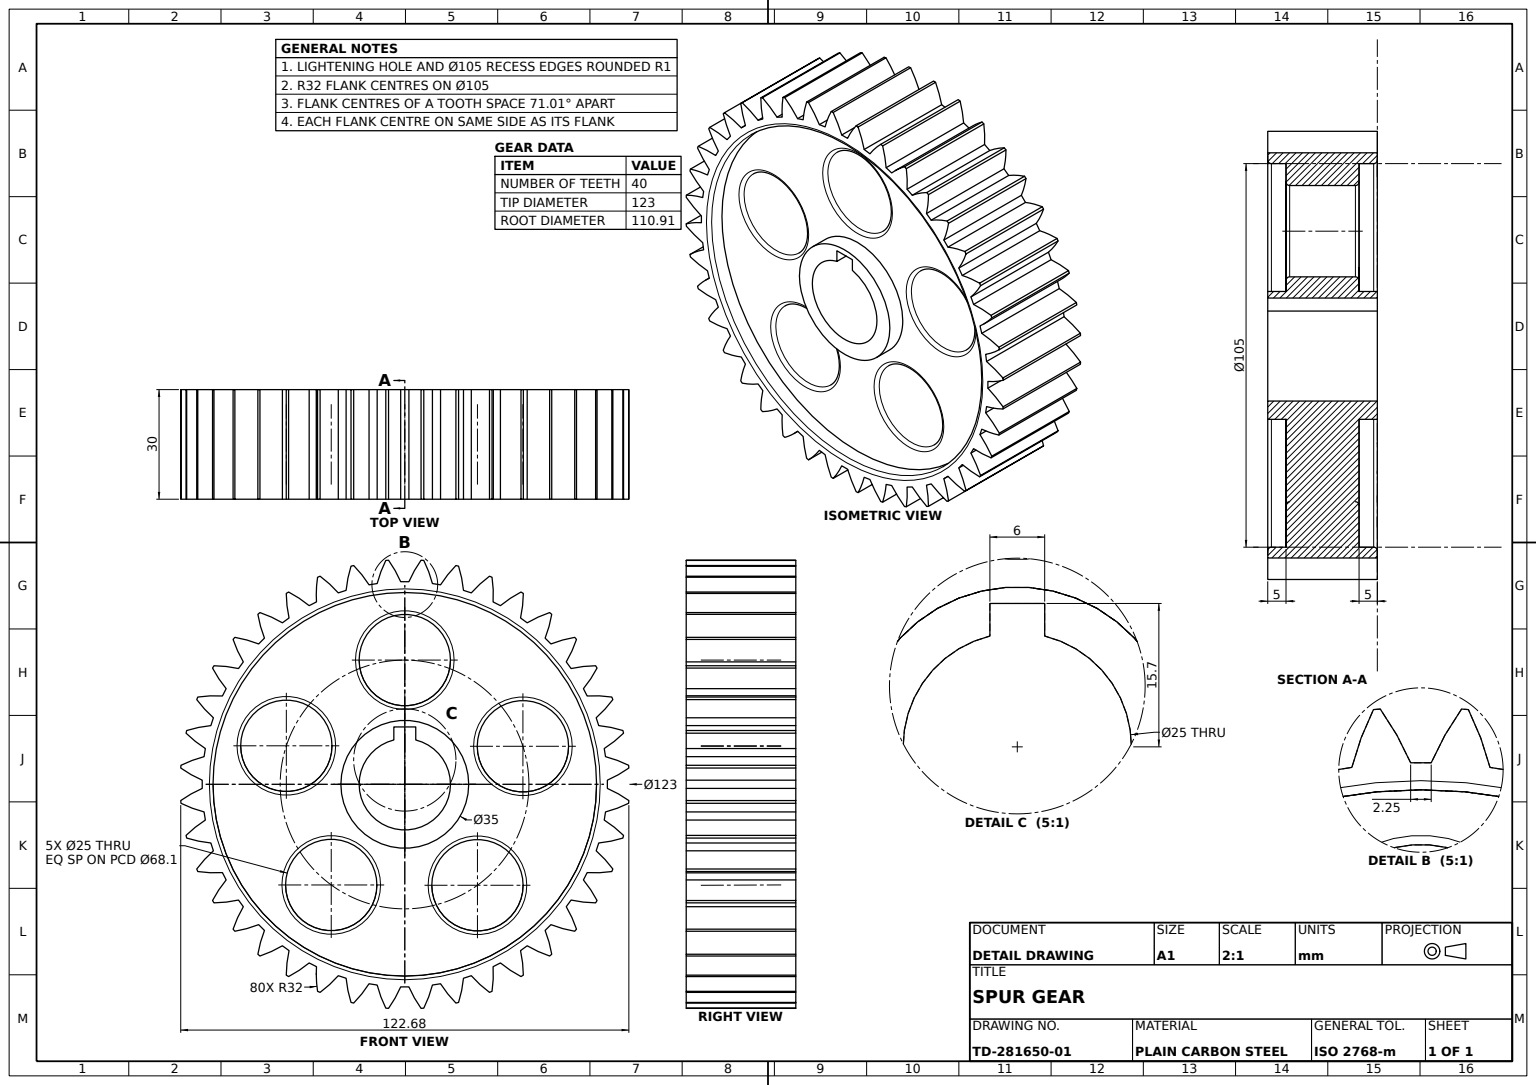
from build123d import *

# Parameters (mm, degrees)
GEAR_BLANK_SKETCH_R           = 61.5
GEAR_BLANK_DEPTH              = 30
FACE_RECESS_SKETCH_R          = 52.5
FACE_RECESS_105_DEPTH         = 5
TOOTH_SPACE_CUT_DEPTH         = 91.495856259
TOOTH_SPACE_PATTERN_40X_COUNT = 40
HUB_BOSS_SKETCH_R             = 17.5
HUB_BOSS_35_DEPTH             = 5
LIGHTENING_HOLES_DEPTH        = 91.276768883
LIGHTENING_HOLES_DEPTH_BACK   = 91.276768883
LIGHTENING_HOLES_SKETCH_R     = 12.5
EDGE_FILLETS_R1_R             = 1


with BuildPart() as part:
    # Gear Blank Sketch → Gear Blank (new body)
    with BuildSketch(Plane.XY):
        Circle(GEAR_BLANK_SKETCH_R)
        with BuildLine():
            Line((-3, 12.1346611), (-3, 15.7))
            Line((-3, 15.7), (3, 15.7))
            Line((3, 15.7), (3, 12.1346611))
            ThreePointArc((3, 12.1346611), (0, -12.5), (-3, 12.1346611))
        make_face(mode=Mode.SUBTRACT)
    extrude(amount=GEAR_BLANK_DEPTH)

    # Face Recess Sketch → Face Recess Ø105 (cut)
    with BuildSketch(Plane.XY.offset(30)):
        Circle(FACE_RECESS_SKETCH_R)
    face_recess_105 = extrude(amount=-FACE_RECESS_105_DEPTH, mode=Mode.SUBTRACT)

    # Face Recess Mirror: Face Recess Ø105 across plane
    add(face_recess_105.mirror(Plane.XY.offset(15)), mode=Mode.SUBTRACT)

    # Tooth Space Sketch → Tooth Space Cut (cut, symmetric)
    with BuildSketch(Plane.XY.offset(25)):
        with BuildLine():
            Line((-1.125, 55.456369197), (1.125, 55.456369197))
            ThreePointArc((1.125, 55.456369197), (2.631798544, 58.485590181), (4.45, 61.338792782))
            ThreePointArc((4.45, 61.338792782), (0, 61.5), (-4.45, 61.338792782))
            ThreePointArc((-4.45, 61.338792782), (-2.631798544, 58.485590181), (-1.125, 55.456369197))
        make_face()
    tooth_space_cut = extrude(amount=TOOTH_SPACE_CUT_DEPTH, both=True, mode=Mode.SUBTRACT)

    # Tooth Space Pattern 40x: Tooth Space Cut ×40 about axis
    tooth_space_pattern_40x_axis = Axis((0, 0, 0), (0, 0, 1))
    for i in range(1, TOOTH_SPACE_PATTERN_40X_COUNT):
        add(tooth_space_cut.rotate(tooth_space_pattern_40x_axis, i * 360 / TOOTH_SPACE_PATTERN_40X_COUNT), mode=Mode.SUBTRACT)

    # Hub Boss Sketch → Hub Boss Ø35 (add)
    with BuildSketch(Plane.XY.offset(25)):
        Circle(HUB_BOSS_SKETCH_R)
        with BuildLine():
            Line((3, 15.7), (-3, 15.7))
            Line((-3, 15.7), (-3, 12.1346611))
            ThreePointArc((-3, 12.1346611), (0, -12.5), (3, 12.1346611))
            Line((3, 12.1346611), (3, 15.7))
        make_face(mode=Mode.SUBTRACT)
    hub_boss_35 = extrude(amount=HUB_BOSS_35_DEPTH)

    # Hub Boss Mirror: Hub Boss Ø35 across plane
    add(hub_boss_35.mirror(Plane.XY.offset(15)))

    # Lightening Holes Sketch → Lightening Holes (cut, two sides: drawn at the far end of the back side and taken through both)
    with BuildSketch(Plane.XY.offset(25).offset(-LIGHTENING_HOLES_DEPTH_BACK)):
        with Locations((0, 34)):
            Circle(LIGHTENING_HOLES_SKETCH_R)
        with Locations((32.431027206, 10.537479508)):
            Circle(LIGHTENING_HOLES_SKETCH_R)
        with Locations((20.138582755, -27.556577809)):
            Circle(LIGHTENING_HOLES_SKETCH_R)
        with Locations((-19.889592926, -27.637479508)):
            Circle(LIGHTENING_HOLES_SKETCH_R)
        with Locations((-32.335921554, 10.406577809)):
            Circle(LIGHTENING_HOLES_SKETCH_R)
    extrude(amount=LIGHTENING_HOLES_DEPTH + LIGHTENING_HOLES_DEPTH_BACK, mode=Mode.SUBTRACT)

    # Edge Fillets R1
    edge_fillets_r1_edges = [part.edges().sort_by_distance(p)[0] for p in [
        (-52.5, 0, 30),
        (-52.5, 0, 0),
        (7.638582755, -27.556577809, 25),
        (7.638582755, -27.556577809, 5),
        (-12.5, 34, 25),
        (-12.5, 34, 5),
        (-32.389592926, -27.637479508, 25),
        (-32.389592926, -27.637479508, 5),
        (-44.835921554, 10.406577809, 25),
        (-44.835921554, 10.406577809, 5),
        (19.931027206, 10.537479508, 25),
        (19.931027206, 10.537479508, 5),
    ]]
    fillet(edge_fillets_r1_edges, radius=EDGE_FILLETS_R1_R)


solid = part.part
